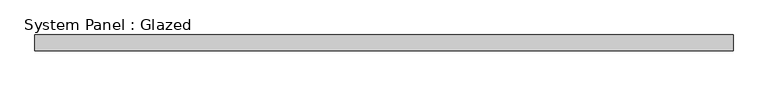
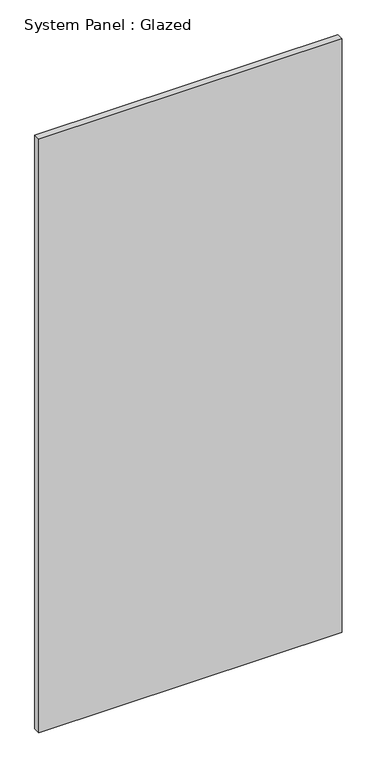
"""IFC4 building model written with IfcOpenShell, lengths in millimetres: plate geometry, System Panel : Glazed."""

from ifc_helpers import new_model, si_unit, origin, origin_with_axes, place, context, project, spatial, polyline, outline, extrude, source, transform, mapped, element, save


def system_panel_glazed_bba99bb7(model_context):
    return source(origin(), model_context, "Body", "SweptSolid", [
        extrude(outline(polyline([(566.2083333, 19.05), (-566.2083333, 19.05), (-566.2083333, 44.45), (566.2083333, 44.45), (566.2083333, 19.05)])), origin_with_axes(), (0.0, 0.0, 1.0), 2343.15),
    ])


if __name__ == "__main__":
    model = new_model("IFC4")
    model_context = context("Model", 3, world=origin())
    ifc_project = project(units=[si_unit("LENGTHUNIT", "METRE", prefix="MILLI")], contexts=[model_context])
    site = spatial("IfcSite", under=ifc_project)
    building = spatial("IfcBuilding", under=site)
    placement = place(None, origin())
    system_panel_glazed_shape = system_panel_glazed_bba99bb7(model_context)
    element("IfcPlate", 1, ObjectType="System Panel : Glazed", at=placement, inside=building, context=model_context, shape_type="MappedRepresentation", body=[
        mapped(system_panel_glazed_shape, transform((0.0, 0.0, 0.0), x_axis=(1.0, 0.0, 0.0), y_axis=(0.0, 1.0, 0.0), z_axis=(0.0, 0.0, 1.0))),
    ])
    save(model, "model.ifc")

# Revit data of these elements
# Type "System Panel : Glazed"
#   Construction Type Id = "GSP4R"
#   Analytic Construction = "1/8 in Pilkington single glazing"
#   Visual Light Transmittance = 0.9
#   Solar Heat Gain Coefficient = 0.86
#   Heat Transfer Coefficient (U) = 1.18115 BTU/(h·ft²·°F)
# Element 1 (IfcPlate, "System Panel : Glazed")
#   Materials on its faces: "Glass"
# Materials
#   "Glass": class "Glass", colour RGB 0 128 192, transparency 0.75, Description = "Soda Lime Glass", Cost = 0
